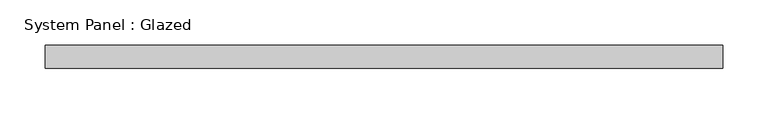
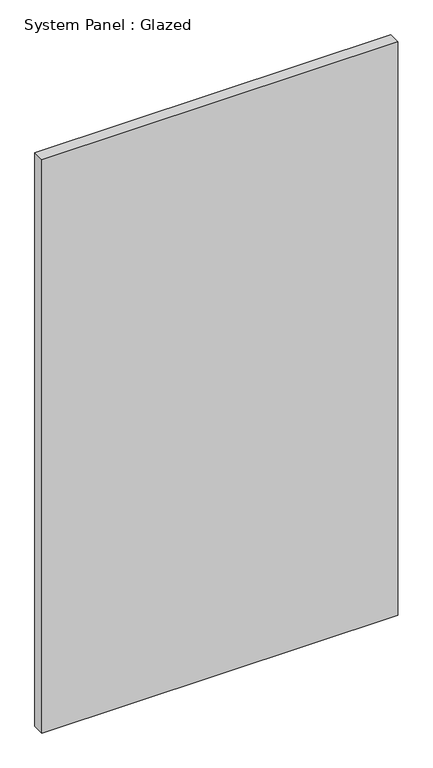
"""IFC4 building model written with IfcOpenShell, lengths in millimetres: plate geometry, System Panel : Glazed."""

from ifc_helpers import new_model, si_unit, origin, origin_with_axes, place, context, project, spatial, polyline, outline, extrude, source, transform, mapped, element, save


def system_panel_glazed_0771ef41(model_context):
    return source(origin(), model_context, "Body", "SweptSolid", [
        extrude(outline(polyline([(374.65, 19.05), (-374.65, 19.05), (-374.65, 44.45), (374.65, 44.45), (374.65, 19.05)])), origin_with_axes(), (0.0, 0.0, 1.0), 1276.35),
    ])


if __name__ == "__main__":
    model = new_model("IFC4")
    model_context = context("Model", 3, world=origin())
    ifc_project = project(units=[si_unit("LENGTHUNIT", "METRE", prefix="MILLI")], contexts=[model_context])
    site = spatial("IfcSite", under=ifc_project)
    building = spatial("IfcBuilding", under=site)
    placement = place(None, origin())
    system_panel_glazed_shape = system_panel_glazed_0771ef41(model_context)
    element("IfcPlate", 1, ObjectType="System Panel : Glazed", at=placement, inside=building, context=model_context, shape_type="MappedRepresentation", body=[
        mapped(system_panel_glazed_shape, transform((0.0, 0.0, 0.0), x_axis=(1.0, 0.0, 0.0), y_axis=(0.0, 1.0, 0.0), z_axis=(0.0, 0.0, 1.0))),
    ])
    save(model, "model.ifc")

# Revit data of these elements
# Type "System Panel : Glazed"
#   Construction Type Id = "GSP4R"
#   Analytic Construction = "1/8 in Pilkington single glazing"
#   Visual Light Transmittance = 0.9
#   Solar Heat Gain Coefficient = 0.86
#   Heat Transfer Coefficient (U) = 1.18115 BTU/(h·ft²·°F)
#   Define Thermal Properties by = 1
# Element 1 (IfcPlate, "System Panel : Glazed")
#   Materials on its faces: "Glass"
# Materials
#   "Glass": class "Glass", colour RGB 0 128 192, transparency 0.75, Description = "Soda Lime Glass", Cost = 0
